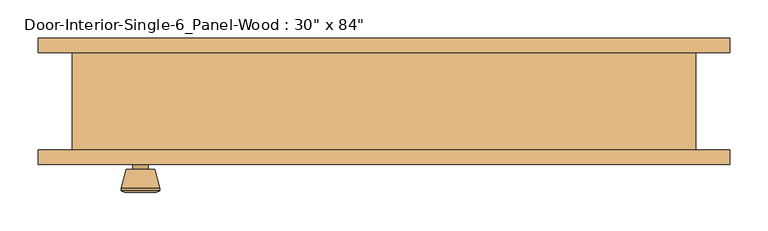
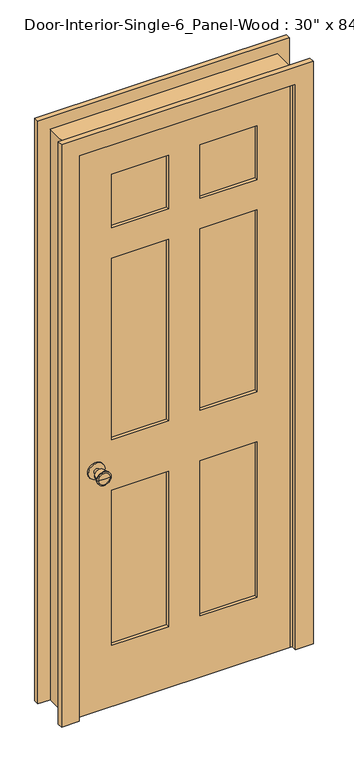
"""IFC4 building model written with IfcOpenShell, lengths in millimetres: door geometry."""

from ifc_helpers import new_model, si_unit, point, frame, frame_2d, origin, place, context, project, spatial, polyline, circle_curve, trimmed, segment, composite_curve, outline, extrude, faceted_brep, source, transform, mapped, element, save
from ifc_brep_helpers import plane_surface, cylinder_surface, revolved_surface, advanced_brep


def door_3b50870b(model_context):
    return source(origin(), model_context, "Body", "SolidModel", [
        advanced_brep(
        [(-317.5, -19.4, 914.4), (-327.5, -19.4, 914.4), (-307.5, -19.4, 914.4), (-297.0241324, 29.6, 914.4), (-337.9758676, 29.6, 914.4), (-317.5, 29.6, 914.4), (-292.5, 27.7721319, 914.4), (-342.5, 27.7721319, 914.4), (-292.5, 24.3084537, 914.4), (-342.5, 24.3084537, 914.4), (-298.863764, -0.4, 914.4), (-336.136236, -0.4, 914.4), (-307.5, -0.4, 914.4), (-327.5, -0.4, 914.4)],
        [
            (0, 1),
            (1, 2, circle_curve(frame((-317.5, -19.4, 914.4), z_axis=(0.0, -1.0, 0.0), x_axis=(-1.0, 0.0, 0.0)), 10.0)),
            (2, 0),
            (2, 1, circle_curve(frame((-317.5, -19.4, 914.4), z_axis=(0.0, -1.0, 0.0), x_axis=(-1.0, 0.0, 0.0)), 10.0)),
            (3, 4, circle_curve(frame((-317.5, 29.6, 914.4), z_axis=(0.0, 1.0, 0.0), x_axis=(-1.0, 0.0, 0.0)), 20.4758676)),
            (4, 5),
            (5, 3),
            (4, 3, circle_curve(frame((-317.5, 29.6, 914.4), z_axis=(0.0, 1.0, 0.0), x_axis=(-1.0, 0.0, 0.0)), 20.4758676)),
            (6, 7, circle_curve(frame((-317.5, 27.7721319, 914.4), z_axis=(0.0, 1.0, 0.0), x_axis=(-1.0, 0.0, 0.0)), 25.0)),
            (7, 4),
            (3, 6),
            (7, 6, circle_curve(frame((-317.5, 27.7721319, 914.4), z_axis=(0.0, 1.0, 0.0), x_axis=(-1.0, 0.0, 0.0)), 25.0)),
            (8, 9, circle_curve(frame((-317.5, 24.3084537, 914.4), z_axis=(0.0, 1.0, 0.0), x_axis=(-1.0, 0.0, 0.0)), 25.0)),
            (9, 7),
            (6, 8),
            (9, 8, circle_curve(frame((-317.5, 24.3084537, 914.4), z_axis=(0.0, 1.0, 0.0), x_axis=(-1.0, 0.0, 0.0)), 25.0)),
            (10, 11, circle_curve(frame((-317.5, -0.4, 914.4), z_axis=(0.0, 1.0, 0.0), x_axis=(-1.0, 0.0, 0.0)), 18.636236)),
            (11, 9),
            (8, 10),
            (11, 10, circle_curve(frame((-317.5, -0.4, 914.4), z_axis=(0.0, 1.0, 0.0), x_axis=(-1.0, 0.0, 0.0)), 18.636236)),
            (12, 13, circle_curve(frame((-317.5, -0.4, 914.4), z_axis=(0.0, 1.0, 0.0), x_axis=(-1.0, 0.0, 0.0)), 10.0)),
            (13, 11),
            (10, 12),
            (13, 12, circle_curve(frame((-317.5, -0.4, 914.4), z_axis=(0.0, 1.0, 0.0), x_axis=(-1.0, 0.0, 0.0)), 10.0)),
            (1, 13),
            (12, 2),
        ],
        [
            plane_surface(frame((-317.5, -19.4, 914.4), z_axis=(0.0, -1.0, 0.0), x_axis=(-1.0, 0.0, 0.0))),
            plane_surface(frame((-317.5, 29.6, 914.4), z_axis=(0.0, 1.0, 0.0), x_axis=(-1.0, 0.0, 0.0))),
            revolved_surface(polyline([(-337.9758676, 29.6, 914.4), (-342.5, 27.7721319, 914.4)]), (-317.5, -19.4, 914.4), (0.0, -1.0, 0.0)),
            cylinder_surface(frame((-317.5, -19.4, 914.4), z_axis=(0.0, -1.0, 0.0), x_axis=(-1.0, 0.0, 0.0)), 25.0),
            revolved_surface(polyline([(-342.5, 24.3084537, 914.4), (-336.136236, -0.4, 914.4)]), (-317.5, -19.4, 914.4), (0.0, -1.0, 0.0)),
            plane_surface(frame((-317.5, -0.4, 914.4), z_axis=(0.0, -1.0, 0.0), x_axis=(-1.0, 0.0, 0.0))),
            cylinder_surface(frame((-317.5, -19.4, 914.4), z_axis=(0.0, -1.0, 0.0), x_axis=(-1.0, 0.0, 0.0)), 10.0),
        ],
        [
            (0, [[1, 2, 3]]),
            (0, [[-3, 4, -1]]),
            (1, [[5, 6, 7]]),
            (1, [[8, -7, -6]]),
            (2, [[9, 10, -5, 11]]),
            (2, [[12, -11, -8, -10]]),
            (3, [[13, 14, -9, 15]]),
            (3, [[16, -15, -12, -14]]),
            (4, [[17, 18, -13, 19]]),
            (4, [[20, -19, -16, -18]]),
            (5, [[21, 22, -17, 23]]),
            (5, [[24, -23, -20, -22]]),
            (6, [[-2, 25, -21, 26]]),
            (6, [[-4, -26, -24, -25]]),
        ],
    ),
        extrude(outline(composite_curve([segment(trimmed(circle_curve(frame_2d((914.4, -317.5)), 30.0), [point((914.4, -347.5))], [point((914.4, -287.5))], False, "CARTESIAN"), True, "CONTINUOUS"), segment(trimmed(circle_curve(frame_2d((914.4, -317.5)), 30.0), [point((914.4, -287.5))], [point((914.4, -347.5))], False, "CARTESIAN"), True, "CONTINUOUS")], self_intersect=False)), frame((0.0, -25.4, 0.0), z_axis=(0.0, 1.0, 0.0), x_axis=(0.0, 0.0, 1.0)), (0.0, 0.0, 1.0), 6.0),
        advanced_brep(
        [(-317.5, -66.325, 914.4), (-307.5, -66.325, 914.4), (-327.5, -66.325, 914.4), (-297.0241324, -115.325, 914.4), (-317.5, -115.325, 914.4), (-337.9758676, -115.325, 914.4), (-292.5, -113.4971319, 914.4), (-342.5, -113.4971319, 914.4), (-292.5, -110.0334537, 914.4), (-342.5, -110.0334537, 914.4), (-298.863764, -85.325, 914.4), (-336.136236, -85.325, 914.4), (-307.5, -85.325, 914.4), (-327.5, -85.325, 914.4)],
        [
            (0, 1),
            (1, 2, circle_curve(frame((-317.5, -66.325, 914.4), z_axis=(0.0, 1.0, 0.0), x_axis=(-1.0, 0.0, 0.0)), 10.0)),
            (2, 0),
            (2, 1, circle_curve(frame((-317.5, -66.325, 914.4), z_axis=(0.0, 1.0, 0.0), x_axis=(-1.0, 0.0, 0.0)), 10.0)),
            (3, 4),
            (4, 5),
            (5, 3, circle_curve(frame((-317.5, -115.325, 914.4), z_axis=(0.0, -1.0, 0.0), x_axis=(-1.0, 0.0, 0.0)), 20.4758676)),
            (3, 5, circle_curve(frame((-317.5, -115.325, 914.4), z_axis=(0.0, -1.0, 0.0), x_axis=(-1.0, 0.0, 0.0)), 20.4758676)),
            (6, 3),
            (5, 7),
            (7, 6, circle_curve(frame((-317.5, -113.4971319, 914.4), z_axis=(0.0, -1.0, 0.0), x_axis=(-1.0, 0.0, 0.0)), 25.0)),
            (6, 7, circle_curve(frame((-317.5, -113.4971319, 914.4), z_axis=(0.0, -1.0, 0.0), x_axis=(-1.0, 0.0, 0.0)), 25.0)),
            (8, 6),
            (7, 9),
            (9, 8, circle_curve(frame((-317.5, -110.0334537, 914.4), z_axis=(0.0, -1.0, 0.0), x_axis=(-1.0, 0.0, 0.0)), 25.0)),
            (8, 9, circle_curve(frame((-317.5, -110.0334537, 914.4), z_axis=(0.0, -1.0, 0.0), x_axis=(-1.0, 0.0, 0.0)), 25.0)),
            (10, 8),
            (9, 11),
            (11, 10, circle_curve(frame((-317.5, -85.325, 914.4), z_axis=(0.0, -1.0, 0.0), x_axis=(-1.0, 0.0, 0.0)), 18.636236)),
            (10, 11, circle_curve(frame((-317.5, -85.325, 914.4), z_axis=(0.0, -1.0, 0.0), x_axis=(-1.0, 0.0, 0.0)), 18.636236)),
            (12, 10),
            (11, 13),
            (13, 12, circle_curve(frame((-317.5, -85.325, 914.4), z_axis=(0.0, -1.0, 0.0), x_axis=(-1.0, 0.0, 0.0)), 10.0)),
            (12, 13, circle_curve(frame((-317.5, -85.325, 914.4), z_axis=(0.0, -1.0, 0.0), x_axis=(-1.0, 0.0, 0.0)), 10.0)),
            (1, 12),
            (13, 2),
        ],
        [
            plane_surface(frame((-317.5, -66.325, 914.4), z_axis=(0.0, 1.0, 0.0), x_axis=(-1.0, 0.0, 0.0))),
            plane_surface(frame((-317.5, -115.325, 914.4), z_axis=(0.0, -1.0, 0.0), x_axis=(-1.0, 0.0, 0.0))),
            revolved_surface(polyline([(-337.9758676, -115.325, 914.4), (-342.5, -113.4971319, 914.4)]), (-317.5, -66.325, 914.4), (0.0, 1.0, 0.0)),
            cylinder_surface(frame((-317.5, -66.325, 914.4), z_axis=(0.0, 1.0, 0.0), x_axis=(-1.0, 0.0, 0.0)), 25.0),
            revolved_surface(polyline([(-342.5, -110.0334537, 914.4), (-336.136236, -85.325, 914.4)]), (-317.5, -66.325, 914.4), (0.0, 1.0, 0.0)),
            plane_surface(frame((-317.5, -85.325, 914.4), z_axis=(0.0, 1.0, 0.0), x_axis=(-1.0, 0.0, 0.0))),
            cylinder_surface(frame((-317.5, -66.325, 914.4), z_axis=(0.0, 1.0, 0.0), x_axis=(-1.0, 0.0, 0.0)), 10.0),
        ],
        [
            (0, [[1, 2, 3]]),
            (0, [[-3, 4, -1]]),
            (1, [[5, 6, 7]]),
            (1, [[-6, -5, 8]]),
            (2, [[9, -7, 10, 11]]),
            (2, [[-10, -8, -9, 12]]),
            (3, [[13, -11, 14, 15]]),
            (3, [[-14, -12, -13, 16]]),
            (4, [[17, -15, 18, 19]]),
            (4, [[-18, -16, -17, 20]]),
            (5, [[21, -19, 22, 23]]),
            (5, [[-22, -20, -21, 24]]),
            (6, [[25, -23, 26, -2]]),
            (6, [[-26, -24, -25, -4]]),
        ],
    ),
        extrude(outline(composite_curve([segment(trimmed(circle_curve(frame_2d((914.4, -317.5)), 30.0), [point((914.4, -347.5))], [point((914.4, -287.5))], False, "CARTESIAN"), True, "CONTINUOUS"), segment(trimmed(circle_curve(frame_2d((914.4, -317.5)), 30.0), [point((914.4, -287.5))], [point((914.4, -347.5))], False, "CARTESIAN"), True, "CONTINUOUS")], self_intersect=False)), frame((0.0, -66.325, 0.0), z_axis=(0.0, 1.0, 0.0), x_axis=(0.0, 0.0, 1.0)), (0.0, 0.0, 1.0), 6.0),
        faceted_brep([(406.4, -60.325, 0.0), (381.0, -60.325, 0.0), (381.0, -25.4, 0.0), (368.3, -25.4, 0.0), (368.3, 9.525, 0.0), (381.0, 9.525, 0.0), (381.0, 66.675, 0.0), (406.4, 66.675, 0.0), (406.4, 66.675, 2159.0), (406.4, -60.325, 2159.0), (381.0, 66.675, 2133.6), (-381.0, 66.675, 2133.6), (-381.0, 66.675, 0.0), (-406.4, 66.675, 0.0), (-406.4, 66.675, 2159.0), (381.0, 9.525, 2133.6), (368.3, 9.525, 2120.9), (-368.3, 9.525, 2120.9), (-368.3, 9.525, 0.0), (-381.0, 9.525, 0.0), (-381.0, 9.525, 2133.6), (368.3, -25.4, 2120.9), (381.0, -25.4, 2133.6), (-381.0, -25.4, 2133.6), (-381.0, -25.4, 0.0), (-368.3, -25.4, 0.0), (-368.3, -25.4, 2120.9), (381.0, -60.325, 2133.6), (-406.4, -60.325, 2159.0), (-406.4, -60.325, 0.0), (-381.0, -60.325, 0.0), (-381.0, -60.325, 2133.6)], [[[0, 1, 2, 3, 4, 5, 6, 7]], [[7, 8, 9, 0]], [[6, 10, 11, 12, 13, 14, 8, 7]], [[5, 15, 10, 6]], [[4, 16, 17, 18, 19, 20, 15, 5]], [[3, 21, 16, 4]], [[2, 22, 23, 24, 25, 26, 21, 3]], [[1, 27, 22, 2]], [[0, 9, 28, 29, 30, 31, 27, 1]], [[8, 14, 28, 9]], [[15, 20, 11, 10]], [[21, 26, 17, 16]], [[27, 31, 23, 22]], [[29, 13, 12, 19, 18, 25, 24, 30]], [[14, 13, 29, 28]], [[20, 19, 12, 11]], [[26, 25, 18, 17]], [[31, 30, 24, 23]]]),
        extrude(outline(polyline([(2133.6, -381.0), (0.0, -381.0), (0.0, 381.0), (2133.6, 381.0), (2133.6, -381.0)]), holes=[polyline([(2014.5375, 57.15), (2014.5375, 260.35), (1811.3375, 260.35), (1811.3375, 57.15), (2014.5375, 57.15)]), polyline([(1697.0375, 260.35), (1009.65, 260.35), (1009.65, 57.15), (1697.0375, 57.15), (1697.0375, 260.35)]), polyline([(1009.65, -57.15), (1009.65, -260.35), (1697.0375, -260.35), (1697.0375, -57.15), (1009.65, -57.15)]), polyline([(1811.3375, -260.35), (2014.5375, -260.35), (2014.5375, -57.15), (1811.3375, -57.15), (1811.3375, -260.35)]), polyline([(819.15, 57.15), (819.15, 260.35), (231.775, 260.35), (231.775, 57.15), (819.15, 57.15)]), polyline([(231.775, -57.15), (231.775, -260.35), (819.15, -260.35), (819.15, -57.15), (231.775, -57.15)])]), frame((0.0, -60.325, 0.0), z_axis=(0.0, 1.0, 0.0), x_axis=(0.0, 0.0, 1.0)), (0.0, 0.0, 1.0), 34.925),
        extrude(outline(polyline([(260.35, -37.0416667), (260.35, -48.6833333), (57.15, -48.6833333), (57.15, -37.0416667), (260.35, -37.0416667)])), frame((0.0, 0.0, 1811.3375), z_axis=(0.0, 0.0, 1.0), x_axis=(1.0, 0.0, 0.0)), (0.0, 0.0, 1.0), 203.2),
        extrude(outline(polyline([(260.35, -37.0416667), (260.35, -48.6833333), (57.15, -48.6833333), (57.15, -37.0416667), (260.35, -37.0416667)])), frame((0.0, 0.0, 1009.65), z_axis=(0.0, 0.0, 1.0), x_axis=(1.0, 0.0, 0.0)), (0.0, 0.0, 1.0), 687.3875),
        extrude(outline(polyline([(-57.15, -37.0416667), (-57.15, -48.6833333), (-260.35, -48.6833333), (-260.35, -37.0416667), (-57.15, -37.0416667)])), frame((0.0, 0.0, 1009.65), z_axis=(0.0, 0.0, 1.0), x_axis=(1.0, 0.0, 0.0)), (0.0, 0.0, 1.0), 687.3875),
        extrude(outline(polyline([(-57.15, -37.0416667), (-57.15, -48.6833333), (-260.35, -48.6833333), (-260.35, -37.0416667), (-57.15, -37.0416667)])), frame((0.0, 0.0, 1811.3375), z_axis=(0.0, 0.0, 1.0), x_axis=(1.0, 0.0, 0.0)), (0.0, 0.0, 1.0), 203.2),
        extrude(outline(polyline([(260.35, -37.0416667), (260.35, -48.6833333), (57.15, -48.6833333), (57.15, -37.0416667), (260.35, -37.0416667)])), frame((0.0, 0.0, 231.775), z_axis=(0.0, 0.0, 1.0), x_axis=(1.0, 0.0, 0.0)), (0.0, 0.0, 1.0), 587.375),
        extrude(outline(polyline([(-57.15, -37.0416667), (-57.15, -48.6833333), (-260.35, -48.6833333), (-260.35, -37.0416667), (-57.15, -37.0416667)])), frame((0.0, 0.0, 231.775), z_axis=(0.0, 0.0, 1.0), x_axis=(1.0, 0.0, 0.0)), (0.0, 0.0, 1.0), 587.375),
        extrude(outline(polyline([(0.0, 450.85), (2203.45, 450.85), (2203.45, -450.85), (0.0, -450.85), (0.0, -387.35), (2139.95, -387.35), (2139.95, 387.35), (0.0, 387.35), (0.0, 450.85)])), frame((0.0, -79.375, 0.0), z_axis=(0.0, 1.0, 0.0), x_axis=(0.0, 0.0, 1.0)), (0.0, 0.0, 1.0), 19.05),
        extrude(outline(polyline([(0.0, 450.85), (2203.45, 450.85), (2203.45, -450.85), (0.0, -450.85), (0.0, -387.35), (2139.95, -387.35), (2139.95, 387.35), (0.0, 387.35), (0.0, 450.85)])), frame((0.0, 66.675, 0.0), z_axis=(0.0, 1.0, 0.0), x_axis=(0.0, 0.0, 1.0)), (0.0, 0.0, 1.0), 19.05),
    ])


if __name__ == "__main__":
    model = new_model("IFC4")
    model_context = context("Model", 3, world=origin())
    ifc_project = project(units=[si_unit("LENGTHUNIT", "METRE", prefix="MILLI")], contexts=[model_context])
    site = spatial("IfcSite", under=ifc_project)
    building = spatial("IfcBuilding", under=site)
    placement = place(None, origin())
    door_shape = door_3b50870b(model_context)
    element("IfcDoor", 1, ObjectType="Door-Interior-Single-6_Panel-Wood : 30\" x 84\"", at=placement, inside=building, context=model_context, shape_type="MappedRepresentation", body=[
        mapped(door_shape, transform((0.0, 0.0, 0.0), x_axis=(1.0, 0.0, 0.0), y_axis=(0.0, 1.0, 0.0), z_axis=(0.0, 0.0, 1.0))),
    ])
    save(model, "model.ifc")

# Revit data of these elements
# Type "Door-Interior-Single-6_Panel-Wood : 30\" x 84\""
#   Type Mark = "9"
#   Assembly Code = "C1020300"
#   Analytic Construction = "Wooden"
#   Top Rail = 0' - 4 11/16"
#   Top Panel = 0' - 8"
#   Thickness = 0' - 1 3/8"
#   Thermal Resistance (R) = 2.5876 (h·ft²·°F)/BTU
#   Swing Angle [instance default] = 90.00°
#   Stiles = 0' - 4 3/4"
#   Rough Width = 2' - 8"
#   Rough Height = 7' - 1"
#   Mullion = 0' - 4 1/2"
#   Lock Rail = 0' - 7 1/2"
#   Intermediate Rail = 0' - 4 1/2"
#   Height = 7' - 0"
#   Width = 2' - 6"
#   Heat Transfer Coefficient (U) = 0.3865 BTU/(h·ft²·°F)
#   Bottom Rail = 0' - 9 1/8"
#   Trim Material = Cherry
#   Panel Material = Cherry
#   Frame Material = Cherry
#   Door Handle Material = Aluminum
#   Visual Light Transmittance = 0
#   Solar Heat Gain Coefficient = 0
#   Wall Closure = (empty or 0)
#   Function = (empty or 0)
# Element 1 (IfcDoor, "Door-Interior-Single-6_Panel-Wood : 30\" x 84\"")
#   Materials on its faces: "Cherry", "Aluminum"
# Materials
#   "Cherry": class "Wood", colour RGB 226 177 128, transparency 0, Description = "Prunus Serotina", Cost = 0
#   "Aluminum": class "Metal", colour RGB 247 247 247, transparency 0, Description = "Aluminum 6061", Cost = 0
